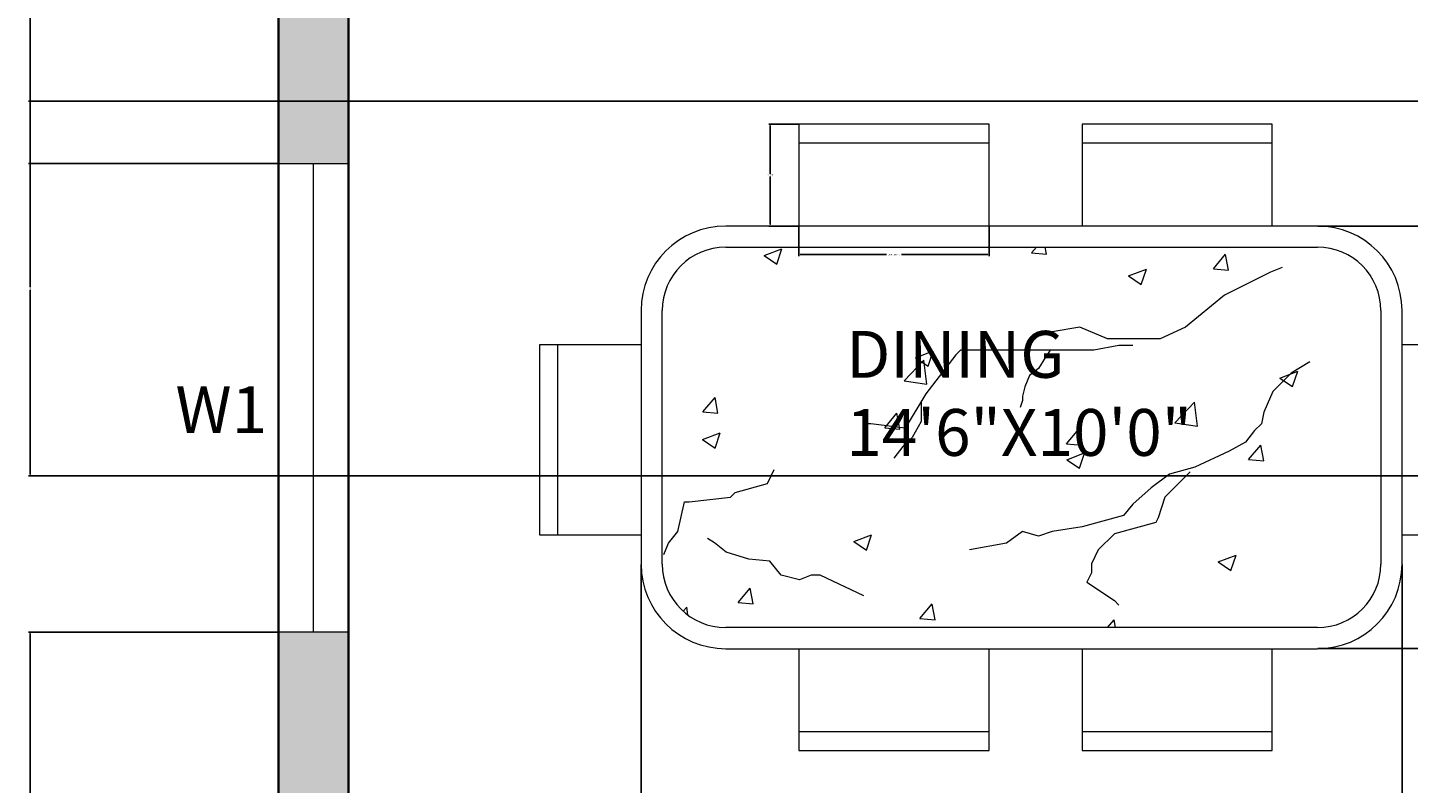
# Model space of a CAD drawing. Units: inches. Extents: x 5 to 421, y -617 to 43.
# Tile 10 of 15: x 5 to 182, y -246 to -149. Entities that reach past the tile are written whole.
import ezdxf

# ---------------------------------------------------------------- set-up
doc = ezdxf.new("R2010")
doc.units = ezdxf.units.IN
doc.header["$MEASUREMENT"] = 0
for name, color, linetype, lineweight in [('A-ANNO-DIMS', 2, 'Continuous', 18), ('A-ANNO-TEXT', 7, 'Continuous', 18), ('A-AREA-IDEN', 7, 'Continuous', 25), ('A-FURN', 8, 'Continuous', 13), ('A-GLAZ', 4, 'Continuous', 18), ('A-WALL', 7, 'Continuous', 35)]:
    doc.layers.add(name, color=color, linetype=linetype, lineweight=lineweight)
doc.layers.add('A-WALL-PATT', color=251, linetype='Continuous', lineweight=13, true_color=0x636466)
doc.styles.get("Standard").update_dxf_attribs({"font": 'arial.ttf'})
doc.dimstyles.get("Standard").update_dxf_attribs({"dimtxt": 0.18, "dimasz": 0.18, "dimexe": 0.18, "dimexo": 0.0625, "dimgap": 0.09, "dimtad": 0, "dimtih": 1, "dimtoh": 1, "dimdec": 0, "dimzin": 0, "dimdsep": 46, "dimlunit": 3, "dimtxsty": 'Standard', "dimcen": 0.09, "dimadec": 0, "dimazin": 0, "dimtfac": 1, "dimtdec": 0, "dimtofl": 0, "dimtmove": 0, "dimatfit": 3, "dimfxl": 1, "dimtolj": 1, "dimtzin": 0, "dimarcsym": 0})

# ---------------------------------------------------------------- blocks, each defined once
blk = doc.blocks.new('WINDOW-W1-60')
for p, q in [((0, 9), (60, 9)), ((0, 0), (0, 9)), ((60, 9), (60, 0)), ((0, 4.5), (60, 4.5)), ((60, 0), (0, 0))]:
    blk.add_line(p, q)
blk = doc.blocks.new('CHAIR-DINING')
for p, q in [((13.04, 24.35), (0, 24.35)), ((10.66, 24.35), (10.66, 0)), ((13.04, 0), (13.04, 24.35)), ((0, 0), (13.04, 0))]:
    blk.add_line(p, q)
blk = doc.blocks.new('*D26')
at = {"layer": 'A-ANNO-DIMS', "color": 0, "lineweight": -2, "transparency": 16777216}
for p, q in [((104.06, -174.69), (104.06, -178.46)), ((128.42, -174.69), (128.42, -178.46)), ((104.24, -178.28), (115.29, -178.28)), ((128.24, -178.28), (117.19, -178.28))]:
    blk.add_line(p, q, dxfattribs=at)
at = {"layer": 'A-ANNO-DIMS', "color": 0, "transparency": 16777216}
for points in [[(104.24, -178.25), (104.24, -178.31), (104.06, -178.28)], [(128.24, -178.25), (128.24, -178.31), (128.42, -178.28)]]:
    blk.add_solid(points, dxfattribs=at)
at = {"layer": 'Defpoints', "color": 0, "transparency": 16777216}
for p in [(104.06, -174.62), (128.42, -174.62), (104.06, -178.28)]:
    blk.add_point(p, dxfattribs=at)
at = {"layer": 'A-ANNO-DIMS', "color": 0, "transparency": 16777216, "insert": (116.24, -178.28), "char_height": 0.18, "attachment_point": 5}
blk.add_mtext('\\A1;CHAIR 24 TYP.', dxfattribs=at)
blk = doc.blocks.new('*D27')
at = {"layer": 'A-ANNO-DIMS', "color": 0, "lineweight": -2, "transparency": 16777216}
for p, q in [((104, -161.58), (100.23, -161.58)), ((100.41, -161.76), (100.41, -167.92)), ((100.41, -174.44), (100.41, -168.28)), ((104, -174.62), (100.23, -174.62))]:
    blk.add_line(p, q, dxfattribs=at)
at = {"layer": 'A-ANNO-DIMS', "color": 0, "transparency": 16777216}
for points in [[(100.38, -161.76), (100.44, -161.76), (100.41, -161.58)], [(100.38, -174.44), (100.44, -174.44), (100.41, -174.62)]]:
    blk.add_solid(points, dxfattribs=at)
at = {"layer": 'Defpoints', "color": 0, "transparency": 16777216}
for p in [(100.41, -161.58), (104.06, -161.58), (104.06, -174.62)]:
    blk.add_point(p, dxfattribs=at)
at = {"layer": 'A-ANNO-DIMS', "color": 0, "transparency": 16777216, "insert": (100.41, -168.1), "char_height": 0.18, "attachment_point": 5}
blk.add_mtext('\\A1;13 TYP.', dxfattribs=at)
blk = doc.blocks.new('*D55')
at = {"layer": 'A-ANNO-DIMS', "color": 0, "lineweight": -2, "transparency": 16777216}
for p, q in [((370.48, 10.88), (420.4, 10.88)), ((420.22, 10.7), (420.22, -286.69)), ((420.22, -584.44), (420.22, -287.05)), ((169.48, -584.62), (420.4, -584.62))]:
    blk.add_line(p, q, dxfattribs=at)
at = {"layer": 'A-ANNO-DIMS', "color": 0, "transparency": 16777216}
for points in [[(420.19, 10.7), (420.25, 10.7), (420.22, 10.88)], [(420.19, -584.44), (420.25, -584.44), (420.22, -584.62)]]:
    blk.add_solid(points, dxfattribs=at)
at = {"layer": 'Defpoints', "color": 0, "transparency": 16777216}
for p in [(370.42, 10.88), (169.42, -584.62), (420.22, -584.62)]:
    blk.add_point(p, dxfattribs=at)
at = {"layer": 'A-ANNO-DIMS', "color": 0, "transparency": 16777216, "insert": (420.22, -286.87), "char_height": 0.18, "attachment_point": 5}
blk.add_mtext('\\A1;595.5', dxfattribs=at)
blk = doc.blocks.new('*D61')
at = {"layer": 'A-ANNO-DIMS', "color": 0, "lineweight": -2, "transparency": 16777216}
for p, q in [((37.36, -88.12), (5.44, -88.12)), ((5.62, -88.3), (5.62, -127.18)), ((5.62, -166.43), (5.62, -127.55)), ((37.36, -166.61), (5.44, -166.61))]:
    blk.add_line(p, q, dxfattribs=at)
at = {"layer": 'A-ANNO-DIMS', "color": 0, "transparency": 16777216}
for points in [[(5.59, -88.3), (5.65, -88.3), (5.62, -88.12)], [(5.59, -166.43), (5.65, -166.43), (5.62, -166.61)]]:
    blk.add_solid(points, dxfattribs=at)
at = {"layer": 'Defpoints', "color": 0, "transparency": 16777216}
for p in [(37.42, -88.12), (5.62, -166.61), (37.42, -166.61)]:
    blk.add_point(p, dxfattribs=at)
at = {"layer": 'A-ANNO-DIMS', "color": 0, "transparency": 16777216, "insert": (5.62, -127.37), "char_height": 0.18, "attachment_point": 5}
blk.add_mtext('\\A1;78.5', dxfattribs=at)
blk = doc.blocks.new('*D62')
at = {"layer": 'A-ANNO-DIMS', "color": 0, "lineweight": -2, "transparency": 16777216}
for p, q in [((37.36, -226.61), (5.44, -226.61)), ((5.62, -226.79), (5.62, -259.52)), ((5.62, -292.62), (5.62, -259.89)), ((37.36, -292.8), (5.44, -292.8))]:
    blk.add_line(p, q, dxfattribs=at)
at = {"layer": 'A-ANNO-DIMS', "color": 0, "transparency": 16777216}
for points in [[(5.59, -226.79), (5.65, -226.79), (5.62, -226.61)], [(5.59, -292.62), (5.65, -292.62), (5.62, -292.8)]]:
    blk.add_solid(points, dxfattribs=at)
at = {"layer": 'Defpoints', "color": 0, "transparency": 16777216}
for p in [(37.42, -226.61), (5.62, -292.8), (37.42, -292.8)]:
    blk.add_point(p, dxfattribs=at)
at = {"layer": 'A-ANNO-DIMS', "color": 0, "transparency": 16777216, "insert": (5.62, -259.71), "char_height": 0.18, "attachment_point": 5}
blk.add_mtext('\\A1;66.19', dxfattribs=at)
blk = doc.blocks.new('*D67')
at = {"layer": 'A-ANNO-DIMS', "color": 0, "lineweight": -2, "transparency": 16777216}
for p, q in [((220.36, -158.62), (5.44, -158.62)), ((5.62, -158.8), (5.62, -182.44)), ((5.62, -206.44), (5.62, -182.8)), ((220.36, -206.62), (5.44, -206.62))]:
    blk.add_line(p, q, dxfattribs=at)
at = {"layer": 'A-ANNO-DIMS', "color": 0, "transparency": 16777216}
for points in [[(5.59, -158.8), (5.65, -158.8), (5.62, -158.62)], [(5.59, -206.44), (5.65, -206.44), (5.62, -206.62)]]:
    blk.add_solid(points, dxfattribs=at)
at = {"layer": 'Defpoints', "color": 0, "transparency": 16777216}
for p in [(220.42, -158.62), (5.62, -206.62), (220.42, -206.62)]:
    blk.add_point(p, dxfattribs=at)
at = {"layer": 'A-ANNO-DIMS', "color": 0, "transparency": 16777216, "insert": (5.62, -182.62), "char_height": 0.18, "attachment_point": 5}
blk.add_mtext('\\A1;48', dxfattribs=at)
blk = doc.blocks.new('*D76')
at = {"layer": 'A-ANNO-DIMS', "color": 0, "lineweight": -2, "transparency": 16777216}
for p, q in [((83.88, -217.98), (83.88, -249.9)), ((181.3, -217.98), (181.3, -249.9)), ((84.06, -249.72), (132.19, -249.72)), ((181.12, -249.72), (132.98, -249.72))]:
    blk.add_line(p, q, dxfattribs=at)
at = {"layer": 'A-ANNO-DIMS', "color": 0, "transparency": 16777216}
for points in [[(84.06, -249.69), (84.06, -249.75), (83.88, -249.72)], [(181.12, -249.69), (181.12, -249.75), (181.3, -249.72)]]:
    blk.add_solid(points, dxfattribs=at)
at = {"layer": 'Defpoints', "color": 0, "transparency": 16777216}
for p in [(83.88, -217.92), (181.3, -217.92), (83.88, -249.72)]:
    blk.add_point(p, dxfattribs=at)
at = {"layer": 'A-ANNO-DIMS', "color": 0, "transparency": 16777216, "insert": (132.59, -249.72), "char_height": 0.18, "attachment_point": 5}
blk.add_mtext('\\A1;97.42', dxfattribs=at)
blk = doc.blocks.new('*D77')
at = {"layer": 'A-ANNO-DIMS', "color": 0, "lineweight": -2, "transparency": 16777216}
for p, q in [((170.53, -174.62), (202.45, -174.62)), ((202.27, -174.8), (202.27, -201.5)), ((202.27, -228.56), (202.27, -201.87)), ((170.53, -228.74), (202.45, -228.74))]:
    blk.add_line(p, q, dxfattribs=at)
at = {"layer": 'A-ANNO-DIMS', "color": 0, "transparency": 16777216}
for points in [[(202.24, -174.8), (202.3, -174.8), (202.27, -174.62)], [(202.24, -228.56), (202.3, -228.56), (202.27, -228.74)]]:
    blk.add_solid(points, dxfattribs=at)
at = {"layer": 'Defpoints', "color": 0, "transparency": 16777216}
for p in [(170.47, -174.62), (170.47, -228.74), (202.27, -228.74)]:
    blk.add_point(p, dxfattribs=at)
at = {"layer": 'A-ANNO-DIMS', "color": 0, "transparency": 16777216, "insert": (202.27, -201.68), "char_height": 0.18, "attachment_point": 5}
blk.add_mtext('\\A1;54.12', dxfattribs=at)

msp = doc.modelspace()

# ---------------------------------------------------------------- hatches: boundary and pattern name
at = {"layer": 'A-WALL-PATT'}
h = msp.add_hatch(color=256, dxfattribs=at)
h.dxf.hatch_style = 1
h.paths.add_polyline_path([(46.4196, -88.1188), (37.4196, -88.1188), (37.4196, -166.6119), (46.4196, -166.6119), (46.4196, -122.6188), (135.4196, -122.6188), (135.4196, -120.3688), (135.4196, -118.1188), (46.4196, -118.1188)])
h.paths.add_polyline_path([(82.4196, 10.8812), (37.4196, 10.8812), (37.4196, -28.1188), (46.4196, -28.1188), (46.4196, 1.8812), (82.4196, 1.8812)])
h.paths.add_polyline_path([(215.5968, 10.8812), (142.4196, 10.8812), (142.4196, 1.8812), (178.4196, 1.8812), (178.4196, -118.1188), (175.4196, -118.1188), (175.4196, -122.6188), (182.9196, -122.6188), (182.9196, -80.6188), (211.9196, -80.6188), (211.9196, -78.3688), (211.9196, -76.1188), (182.9196, -76.1188), (182.9196, 1.8812), (215.5968, 1.8812)])
h.paths.add_polyline_path([(274.4196, 10.8812), (239.5968, 10.8812), (239.5968, 1.8812), (242.9196, 1.8812), (242.9196, -76.1188), (239.9196, -76.1188), (239.9196, -80.6188), (242.9196, -80.6188), (242.9196, -83.6188), (247.4196, -83.6188), (247.4196, 1.8812), (274.4196, 1.8812)])
h.paths.add_polyline_path([(370.4196, 10.8812), (334.4196, 10.8812), (334.4196, 1.8812), (361.4196, 1.8812), (361.4196, -28.1188), (370.4196, -28.1188)])
h.paths.add_polyline_path([(370.4196, -88.1188), (361.4196, -88.1188), (361.4196, -118.1188), (247.4196, -118.1188), (247.4196, -115.1188), (242.9196, -115.1188), (242.9196, -118.1188), (220.4196, -118.1188), (220.4196, -158.6188), (224.9196, -158.6188), (224.9196, -122.6188), (326.9196, -122.6188), (326.9196, -170.7662), (331.4196, -170.7662), (331.4196, -122.6188), (370.4196, -122.6188)])
h.paths.add_polyline_path([(388.4196, -122.6188), (388.4196, -118.1188), (379.4196, -118.1188), (379.4196, -122.6188), (379.4196, -154.8688), (388.4196, -154.8688)])
h.paths.add_polyline_path([(388.4196, -214.8688), (379.4196, -214.8688), (379.4196, -247.1188), (388.4196, -247.1188)])
h.paths.add_polyline_path([(371.0265, -242.6188), (331.4196, -242.6188), (331.4196, -239.6188), (326.9196, -239.6188), (326.9196, -242.6188), (224.9196, -242.6188), (224.9196, -206.6188), (220.4196, -206.6188), (220.4196, -343.6188), (224.9196, -343.6188), (229.4196, -343.6188), (229.4196, -247.1188), (261.5265, -247.1188), (261.5265, -276.1188), (263.7765, -276.1188), (266.0265, -276.1188), (266.0265, -247.1188), (362.0265, -247.1188), (362.0265, -265.1188), (371.0265, -265.1188), (371.0265, -247.1188)])
h.paths.add_polyline_path([(371.0265, -289.1188), (362.0265, -289.1188), (362.0265, -307.1188), (266.0265, -307.1188), (266.0265, -304.1188), (261.5265, -304.1188), (261.5265, -307.1188), (261.5265, -311.6188), (362.0265, -311.6188), (362.0265, -353.6188), (371.0265, -353.6188)])
h.paths.add_polyline_path([(371.0265, -413.6188), (362.0265, -413.6188), (362.0265, -455.6188), (325.7231, -455.6188), (325.7231, -464.6188), (361.4196, -464.6188), (371.0265, -464.6188)])
h.paths.add_polyline_path([(265.7231, -455.6188), (229.4196, -455.6188), (229.4196, -383.6188), (220.4196, -383.6188), (220.4196, -386.6188), (207.4649, -386.6188), (207.4649, -395.6188), (220.4196, -395.6188), (220.4196, -455.6188), (216.0568, -455.6188), (216.0568, -464.6188), (265.7231, -464.6188)])
h.paths.add_polyline_path([(169.4196, -386.6188), (137.9196, -386.6188), (137.9196, -395.6188), (160.4196, -395.6188), (160.4196, -424.2032), (169.4196, -424.2032)])
h.paths.add_polyline_path([(169.4196, -453.7423), (160.4196, -453.7423), (160.4196, -464.6188), (169.4196, -464.6188)])
h.paths.add_polyline_path([(46.4196, -575.6188), (37.4196, -575.6188), (37.4196, -584.6188), (46.4196, -584.6188)])
h.paths.add_polyline_path([(169.4196, -575.6188), (160.4196, -575.6188), (160.4196, -579.5504), (160.4196, -584.6188), (169.4196, -584.6188)])
h.paths.add_polyline_path([(46.4196, -226.6119), (37.4196, -226.6119), (37.4196, -292.8008), (46.4196, -292.8008)])
h.paths.add_polyline_path([(46.4196, -352.8008), (37.4196, -352.8008), (37.4196, -395.6188), (77.9196, -395.6188), (77.9196, -386.6188), (46.4196, -386.6188)])

# ---------------------------------------------------------------- linework, layer by layer
at = {"layer": 'A-FURN'}
for p, q in [((170.4715, -174.6231), (94.7009, -174.6231)), ((94.7009, -177.3292), (170.4715, -177.3292)), ((99.6172, -178.4106), (101.8909, -177.5378)), ((99.6172, -178.4106), (101.2324, -179.5001)), ((101.2327, -179.5014), (101.8911, -177.539)), ((133.8467, -178.074), (134.4717, -177.3292)), ((133.8467, -178.074), (135.7877, -178.2438)), ((135.7879, -178.2451), (135.6189, -177.3292)), ((157.1384, -180.1118), (158.7039, -178.2461)), ((159.0796, -180.2829), (158.7041, -178.2474)), ((146.2852, -181.0113), (148.5589, -180.1385)), ((147.9007, -182.1021), (148.5592, -180.1398)), ((157.1384, -180.1118), (159.0793, -180.2816)), ((165.9402, -179.9479), (164.4689, -180.5357)), ((146.2852, -181.0113), (147.9005, -182.1008)), ((164.4689, -180.5357), (158.5839, -183.4748)), ((158.5839, -183.4748), (153.5817, -187.5895)), ((83.8765, -185.4475), (83.8765, -217.9206)), ((86.5826, -217.9206), (86.5826, -185.4475)), ((178.5898, -185.4475), (178.5898, -217.9206)), ((181.2958, -217.9206), (181.2958, -185.4475)), ((136.5152, -188.1773), (135.3382, -188.4712)), ((140.0462, -187.5895), (136.5152, -188.1773)), ((143.5772, -189.0591), (140.0462, -187.5895)), ((150.3449, -189.0591), (143.5772, -189.0591)), ((153.5817, -187.5895), (150.3449, -189.0591)), ((119.0006, -191.4848), (121.2743, -190.612)), ((120.6161, -192.5757), (121.2745, -190.6133)), ((124.7452, -190.5286), (124.1567, -191.1164)), ((141.8117, -190.5286), (124.7452, -190.5286)), ((136.2251, -190.518), (135.6366, -191.3997)), ((145.0484, -189.9408), (141.8117, -190.5286)), ((146.8139, -189.9408), (145.0484, -189.9408)), ((117.5409, -194.4364), (120.0702, -191.8003)), ((119.0006, -191.4848), (120.6159, -192.5744)), ((120.4291, -194.8854), (120.0704, -191.8014)), ((124.1567, -191.1164), (120.3314, -196.1129)), ((135.6366, -191.3997), (134.7538, -192.8692)), ((169.4712, -191.9981), (167.1172, -193.4677)), ((117.5409, -194.4364), (120.4289, -194.8843)), ((133.5768, -193.751), (132.9883, -195.2205)), ((134.7538, -192.8692), (133.5768, -193.751)), ((167.1172, -193.4677), (164.7632, -195.819)), ((165.6686, -194.0855), (167.9424, -193.2127)), ((165.6686, -194.0855), (167.2839, -195.1751)), ((167.2841, -195.1764), (167.9426, -193.2141)), ((120.3314, -196.1129), (117.6832, -200.5215)), ((132.9883, -195.2205), (132.6941, -196.3961)), ((164.7632, -195.819), (163.5862, -198.4641)), ((91.7691, -198.4245), (93.3346, -196.5588)), ((93.7102, -198.5956), (93.3348, -196.5601)), ((119.7429, -196.9946), (119.7429, -199.6398)), ((132.6941, -196.984), (132.3998, -197.8657)), ((132.6941, -196.3961), (132.6941, -196.984)), ((152.1975, -199.8113), (154.7268, -197.1752)), ((155.0858, -200.2603), (154.727, -197.1764)), ((91.7691, -198.4245), (93.71, -198.5943)), ((115.0607, -200.4623), (116.6262, -198.5966)), ((117.0019, -200.6334), (116.6264, -198.5979)), ((119.7429, -199.6398), (118.5659, -201.6971)), ((163.5862, -198.4641), (163.2919, -199.9337)), ((91.716, -201.9584), (93.9897, -201.0856)), ((93.3314, -203.0492), (93.9899, -201.0869)), ((113.2694, -199.9337), (112.3867, -199.9337)), ((117.6832, -200.5215), (113.2694, -199.9337)), ((115.0607, -200.4623), (117.0017, -200.6321)), ((138.3524, -202.5), (139.9179, -200.6343)), ((140.2936, -202.6712), (139.9181, -200.6357)), ((152.1975, -199.8113), (155.0856, -200.2592)), ((162.4092, -200.8154), (161.2322, -202.285)), ((163.2919, -199.9337), (162.4092, -200.8154)), ((91.716, -201.9584), (93.3312, -203.048)), ((117.3889, -202.8728), (116.2119, -204.3423)), ((118.5659, -201.6971), (117.3889, -202.8728)), ((138.3524, -202.5), (140.2934, -202.6698)), ((161.2322, -202.285), (159.1724, -203.4606)), ((161.6441, -204.5378), (163.2096, -202.6721)), ((163.5852, -204.7089), (163.2098, -202.6734)), ((138.384, -204.5591), (140.6577, -203.6863)), ((138.384, -204.5591), (139.9993, -205.6487)), ((139.9995, -205.65), (140.6579, -203.6876)), ((159.1724, -203.4606), (154.7587, -205.5179)), ((161.6441, -204.5378), (163.585, -204.7076)), ((100.0281, -207.5753), (100.9109, -205.8119)), ((151.5219, -206.3997), (149.1679, -208.1631)), ((154.7587, -205.5179), (151.5219, -206.3997)), ((154.1702, -206.1058), (152.9932, -207.2814)), ((95.9086, -208.7509), (100.0281, -207.5753)), ((149.1679, -208.1631), (146.8139, -210.2205)), ((152.9932, -207.2814), (150.9334, -209.3388)), ((88.5524, -213.7474), (89.4351, -209.9266)), ((89.4351, -209.9266), (90.0236, -209.9266)), ((90.0236, -209.9266), (95.3201, -209.3388)), ((95.3201, -209.3388), (95.9086, -208.7509)), ((146.8139, -210.2205), (145.6369, -211.69)), ((150.9334, -209.3388), (150.0507, -211.9839)), ((145.6369, -211.69), (140.3404, -213.1596)), ((150.0507, -211.9839), (149.7564, -212.5718)), ((87.3754, -215.2169), (88.5524, -213.7474)), ((132.6899, -213.7474), (130.6302, -215.2169)), ((134.7497, -214.3352), (132.6899, -213.7474)), ((136.5152, -213.7474), (134.7497, -214.3352)), ((140.3404, -213.1596), (136.5152, -213.7474)), ((149.7564, -212.5718), (144.4599, -214.0413)), ((86.7869, -216.6865), (87.3754, -215.2169)), ((93.2646, -215.2063), (92.3818, -214.6185)), ((94.7358, -216.3819), (93.2646, -215.2063)), ((111.0994, -215.0327), (113.3731, -214.1599)), ((111.0994, -215.0327), (112.7147, -216.1222)), ((112.7149, -216.1235), (113.3733, -214.1612)), ((130.6302, -215.2169), (125.9222, -216.0987)), ((144.4599, -214.0413), (142.4002, -216.0987)), ((97.6783, -217.2637), (94.7358, -216.3819)), ((100.3266, -217.5576), (97.6783, -217.2637)), ((142.4002, -216.0987), (141.5174, -217.8621)), ((157.7674, -217.6334), (160.0412, -216.7606)), ((159.3829, -218.7243), (160.0414, -216.7619)), ((101.7978, -219.321), (100.3266, -217.5576)), ((141.5174, -219.0377), (140.9289, -220.2134)), ((141.5174, -217.8621), (141.5174, -219.0377)), ((157.7674, -217.6334), (159.3827, -218.7229)), ((96.2747, -222.8505), (97.8402, -220.9848)), ((98.2159, -223.0216), (97.8404, -220.9861)), ((104.1518, -219.9088), (101.7978, -219.321)), ((105.6231, -219.321), (104.1518, -219.9088)), ((106.8001, -219.321), (105.6231, -219.321)), ((112.3908, -221.9662), (106.8001, -219.321)), ((140.9289, -220.2134), (144.4599, -222.5646)), ((144.4599, -222.5646), (145.0484, -223.1525)), ((89.2422, -223.9297), (89.7188, -223.433)), ((89.8334, -224.4178), (89.719, -223.4341)), ((96.2747, -222.8505), (98.2157, -223.0203)), ((119.5664, -224.8883), (121.1319, -223.0226)), ((121.5076, -225.0594), (121.1321, -223.0239)), ((170.4715, -226.0389), (94.7009, -226.0389)), ((119.5664, -224.8883), (121.5074, -225.0581)), ((143.6025, -226.0389), (144.4236, -225.0603)), ((144.604, -226.0389), (144.4238, -225.0617)), ((94.7009, -228.745), (170.4715, -228.745))]:
    msp.add_line(p, q, dxfattribs=at)
for centre, radius, start, end in [((94.7009, -185.4475), 10.8244, 90, 180), ((170.4715, -185.4475), 10.8244, 0, 90), ((94.7009, -185.4475), 8.1183, 90, 180), ((170.4715, -185.4475), 8.1183, 0, 90), ((94.7009, -217.9206), 10.8244, 180, 270), ((94.7009, -217.9206), 8.1183, 180, 270), ((170.4715, -217.9206), 8.1183, 270, 0), ((170.4715, -217.9206), 10.8244, 270, 0)]:
    msp.add_arc(centre, radius, start, end, dxfattribs=at)
at = {"layer": 'A-WALL'}
for p, q in [((37.4196, 10.8812), (37.4196, -584.6188)), ((46.4196, -122.6188), (46.4196, -386.6188))]:
    msp.add_line(p, q, dxfattribs=at)

# ---------------------------------------------------------------- block references
at = {"layer": 'A-FURN'}
for p, rotation in [((128.4188, -174.6231), 89.99999998729199), ((164.6804, -174.6231), 89.99999998729149), ((83.8765, -189.8313), 180), ((104.064, -228.745), 269.9999999884725), ((140.3256, -228.745), 269.9999999884721)]:
    msp.add_blockref('CHAIR-DINING', p, dxfattribs=dict(at, rotation=rotation))
msp.add_blockref('CHAIR-DINING', (181.2958, -214.1862), dxfattribs=at)
at = {"layer": 'A-GLAZ', "rotation": 90.00000000000003}
msp.add_blockref('WINDOW-W1-60', (46.4196, -226.6119), dxfattribs=at)

# ---------------------------------------------------------------- texts
at = {"layer": 'A-ANNO-TEXT', "insert": (24.2415, -195.1415), "char_height": 6, "attachment_point": 1}
msp.add_mtext('W1', dxfattribs=at)
at = {"layer": 'A-AREA-IDEN', "insert": (110.1467, -188.0556), "char_height": 6, "attachment_point": 1}
msp.add_mtext('DINING\\P14\'6"X10\'0"', dxfattribs=at)

# ---------------------------------------------------------------- dimensions: what is measured, and where the dimension line sits
at = {"layer": 'A-ANNO-DIMS'}
for base, p1, p2, angle, override, picture, middle in [((420.2196, -584.6188), (370.4196, 10.8812), (169.4196, -584.6188), 90, {"dimdec": 1, "dimlfac": 1, "dimrnd": 0, "dimzin": 0, "dimdsep": 46, "dimlunit": 2}, '*D55', (420.2196, -286.8688)), ((5.6196, -166.6119), (37.4196, -88.1188), (37.4196, -166.6119), 90, {"dimdec": 1, "dimlfac": 1, "dimrnd": 0, "dimzin": 0, "dimdsep": 46, "dimlunit": 2}, '*D61', (5.6196, -127.3654)), ((5.6196, -206.6188), (220.4196, -158.6188), (220.4196, -206.6188), 90, {"dimdec": 0, "dimlfac": 1, "dimrnd": 0, "dimzin": 0, "dimdsep": 46, "dimlunit": 2}, '*D67', (5.6196, -182.6188)), ((202.2715, -228.745), (170.4715, -174.6231), (170.4715, -228.745), 270, {"dimdec": 2, "dimlfac": 1, "dimrnd": 0, "dimzin": 0, "dimdsep": 46, "dimlunit": 2}, '*D77', (202.2715, -201.684)), ((83.8765, -249.7206), (181.2958, -217.9206), (83.8765, -217.9206), 180, {"dimdec": 2, "dimlfac": 1, "dimrnd": 0, "dimzin": 0, "dimdsep": 46, "dimlunit": 2}, '*D76', (132.5862, -249.7206)), ((5.6196, -292.8008), (37.4196, -226.6119), (37.4196, -292.8008), 90, {"dimdec": 2, "dimlfac": 1, "dimrnd": 0, "dimzin": 0, "dimdsep": 46, "dimlunit": 2}, '*D62', (5.6196, -259.7064))]:
    dim = msp.add_linear_dim(base=base, p1=p1, p2=p2, angle=angle, dimstyle='Standard', override=override, dxfattribs=at)
    dim.commit()
    dim.dimension.update_dxf_attribs({"geometry": picture, "text_midpoint": middle})
for base, p1, p2, angle, text, picture, middle in [((100.4107, -161.5797), (104.064, -174.6231), (104.064, -161.5797), 90, '<> TYP.', '*D27', (100.4107, -168.1014)), ((104.064, -178.2763), (128.4188, -174.6231), (104.064, -174.6231), 180, 'CHAIR <> TYP.', '*D26', (116.2414, -178.2763))]:
    dim = msp.add_linear_dim(base=base, p1=p1, p2=p2, angle=angle, text=text, dimstyle='Standard', override={"dimdec": 0, "dimlfac": 1, "dimrnd": 0, "dimzin": 0, "dimdsep": 46, "dimlunit": 2}, dxfattribs=at)
    dim.commit()
    dim.dimension.update_dxf_attribs({"geometry": picture, "text_midpoint": middle})

doc.saveas('drawing.dxf')
